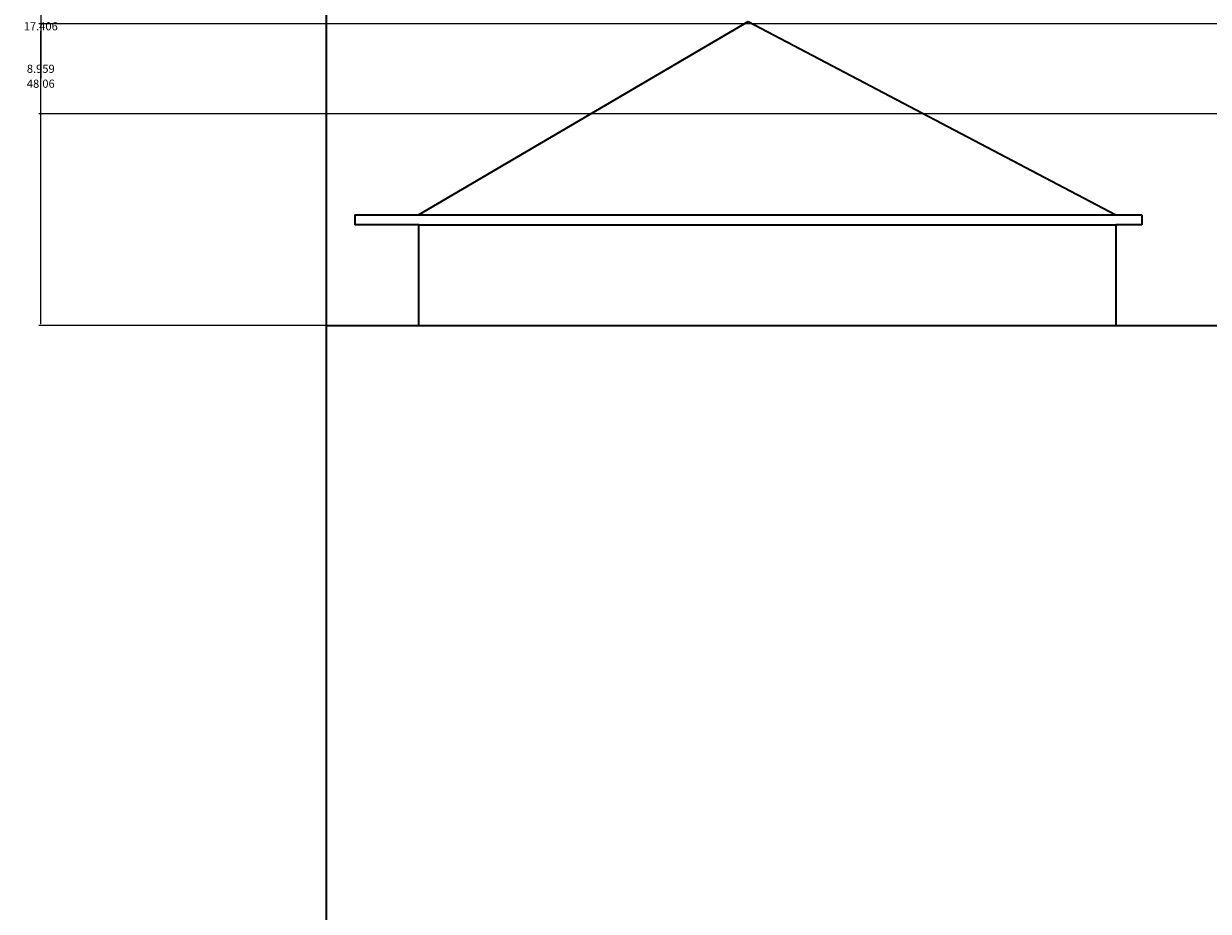
# Model space of a CAD drawing. Units: inches. Extents: x 69 to 650, y -16 to 573.
# Tile 12 of 26: x 69 to 187, y 306 to 394. Entities that reach past the tile are written whole.
import ezdxf

# ---------------------------------------------------------------- set-up
doc = ezdxf.new("R2010")
doc.units = ezdxf.units.IN
doc.header["$MEASUREMENT"] = 0
for name, color, linetype, lineweight in [('A-ANNO-DIMS', 2, 'Continuous', 18), ('A-ROOF', 7, 'Continuous', 35), ('A-WALL', 7, 'Continuous', 35)]:
    doc.layers.add(name, color=color, linetype=linetype, lineweight=lineweight)
doc.styles.get("Standard").update_dxf_attribs({"font": 'arial.ttf'})
doc.dimstyles.get("Standard").update_dxf_attribs({"dimtxt": 0.8125, "dimasz": 0.18, "dimexe": 0.18, "dimexo": 0.0625, "dimgap": 0.09, "dimtad": 0, "dimtih": 1, "dimtoh": 1, "dimdec": 4, "dimzin": 0, "dimdsep": 46, "dimlunit": 4, "dimtxsty": 'Standard', "dimcen": 0.09, "dimadec": 0, "dimazin": 0, "dimtfac": 1, "dimtdec": 4, "dimtofl": 0, "dimtmove": 0, "dimatfit": 3, "dimfxl": 1, "dimtolj": 1, "dimtzin": 0, "dimarcsym": 0})

# ---------------------------------------------------------------- blocks, each defined once
blk = doc.blocks.new('CAP-SIDE-PEDIMENT')
for p, q in [((39.09, 30.19), (2.58, 11)), ((71.85, 11), (39.09, 30.19)), ((78.18, 11), (0, 11)), ((0, 11), (0, 9.99)), ((0, 9.99), (2.58, 9.99)), ((71.82, 9.99), (2.58, 9.99)), ((2.58, 9.99), (2.58, 0)), ((71.82, 0), (71.82, 9.99)), ((71.82, 9.99), (78.18, 9.99))]:
    blk.add_line(p, q)
blk = doc.blocks.new('*D19')
at = {"layer": 'A-ANNO-DIMS', "color": 0, "lineweight": -2, "transparency": 16777216}
for p, q in [((99.56, 471.72), (99.56, 572.74)), ((99.74, 572.56), (358.57, 572.56)), ((619.38, 572.56), (360.54, 572.56)), ((619.56, 87.99), (619.56, 572.74))]:
    blk.add_line(p, q, dxfattribs=at)
at = {"layer": 'A-ANNO-DIMS', "color": 0, "transparency": 16777216}
for points in [[(99.74, 572.59), (99.74, 572.53), (99.56, 572.56)], [(619.38, 572.59), (619.38, 572.53), (619.56, 572.56)]]:
    blk.add_solid(points, dxfattribs=at)
at = {"layer": 'Defpoints', "color": 0, "transparency": 16777216}
for p in [(619.56, 572.56), (99.56, 471.66), (619.56, 87.93)]:
    blk.add_point(p, dxfattribs=at)
at = {"layer": 'A-ANNO-DIMS', "color": 0, "transparency": 16777216, "insert": (359.56, 572.56), "char_height": 0.812, "attachment_point": 5}
blk.add_mtext('\\A1;520', dxfattribs=at)
blk = doc.blocks.new('*D47')
at = {"layer": 'A-ANNO-DIMS', "color": 0, "lineweight": -2, "transparency": 16777216}
for p, q in [((99.49, 411.93), (70.98, 411.93)), ((71.16, 411.75), (71.16, 388.41)), ((71.16, 364.05), (71.16, 387.4)), ((99.49, 363.87), (70.98, 363.87))]:
    blk.add_line(p, q, dxfattribs=at)
at = {"layer": 'A-ANNO-DIMS', "color": 0, "transparency": 16777216}
for points in [[(71.13, 411.75), (71.19, 411.75), (71.16, 411.93)], [(71.13, 364.05), (71.19, 364.05), (71.16, 363.87)]]:
    blk.add_solid(points, dxfattribs=at)
at = {"layer": 'Defpoints', "color": 0, "transparency": 16777216}
for p in [(71.16, 411.93), (99.56, 411.93), (99.56, 363.87)]:
    blk.add_point(p, dxfattribs=at)
at = {"layer": 'A-ANNO-DIMS', "color": 0, "transparency": 16777216, "insert": (71.16, 387.9), "char_height": 0.812, "attachment_point": 5}
blk.add_mtext('\\A1;48.06', dxfattribs=at)
blk = doc.blocks.new('*D59')
at = {"layer": 'A-ANNO-DIMS', "color": 0, "lineweight": -2, "transparency": 16777216}
for p, q in [((214.82, 402.3), (70.98, 402.3)), ((71.16, 402.12), (71.16, 394.11)), ((71.16, 385.08), (71.16, 393.1)), ((307.73, 384.9), (70.98, 384.9))]:
    blk.add_line(p, q, dxfattribs=at)
at = {"layer": 'A-ANNO-DIMS', "color": 0, "transparency": 16777216}
for points in [[(71.13, 402.12), (71.19, 402.12), (71.16, 402.3)], [(71.13, 385.08), (71.19, 385.08), (71.16, 384.9)]]:
    blk.add_solid(points, dxfattribs=at)
at = {"layer": 'Defpoints', "color": 0, "transparency": 16777216}
for p in [(71.16, 402.3), (214.89, 402.3), (307.8, 384.9)]:
    blk.add_point(p, dxfattribs=at)
at = {"layer": 'A-ANNO-DIMS', "color": 0, "transparency": 16777216, "insert": (71.16, 393.6), "char_height": 0.812, "attachment_point": 5}
blk.add_mtext('\\A1;17.406', dxfattribs=at)
blk = doc.blocks.new('*D63')
at = {"layer": 'A-ANNO-DIMS', "color": 0, "lineweight": -2, "transparency": 16777216}
for p, q in [((319.49, 393.86), (70.98, 393.86)), ((71.16, 393.68), (71.16, 389.88)), ((71.16, 385.08), (71.16, 388.87)), ((307.73, 384.9), (70.98, 384.9))]:
    blk.add_line(p, q, dxfattribs=at)
at = {"layer": 'A-ANNO-DIMS', "color": 0, "transparency": 16777216}
for points in [[(71.13, 393.68), (71.19, 393.68), (71.16, 393.86)], [(71.13, 385.08), (71.19, 385.08), (71.16, 384.9)]]:
    blk.add_solid(points, dxfattribs=at)
at = {"layer": 'Defpoints', "color": 0, "transparency": 16777216}
for p in [(71.16, 393.86), (319.55, 393.86), (307.8, 384.9)]:
    blk.add_point(p, dxfattribs=at)
at = {"layer": 'A-ANNO-DIMS', "color": 0, "transparency": 16777216, "insert": (71.16, 389.38), "char_height": 0.812, "attachment_point": 5}
blk.add_mtext('\\A1;8.959', dxfattribs=at)

msp = doc.modelspace()

# ---------------------------------------------------------------- linework, layer by layer
at = {"layer": 'A-ROOF'}
msp.add_line((102.3654, 374.8764), (102.3654, 373.8686), dxfattribs=at)
at = {"layer": 'A-WALL'}
msp.add_line((99.556, 243.93), (99.556, 411.93), dxfattribs=at)
msp.add_lwpolyline([(99.556, 363.8739), (190.299, 363.8739), (190.299, 243.93), (99.556, 243.93)], close=True, dxfattribs=at)

# ---------------------------------------------------------------- block references
at = {"layer": 'A-ROOF', "extrusion": (0, 0, -1), "zscale": -1}
msp.add_blockref('CAP-SIDE-PEDIMENT', (-180.548, 363.874), dxfattribs=at)

# ---------------------------------------------------------------- dimensions: what is measured, and where the dimension line sits
at = {"layer": 'A-ANNO-DIMS'}
dim = msp.add_linear_dim(base=(619.555, 572.5573), p1=(99.556, 471.6595), p2=(619.555, 87.93), dimstyle='Standard', override={"dimdec": 0, "dimlfac": 1, "dimrnd": 0, "dimzin": 0, "dimdsep": 46, "dimlunit": 2}, dxfattribs=at)
dim.commit()
dim.dimension.update_dxf_attribs({"geometry": '*D19', "text_midpoint": (359.5555, 572.5573)})
for base, p1, p2, override, picture, middle in [((71.156, 411.93), (99.556, 363.8739), (99.556, 411.93), {"dimdec": 2, "dimlfac": 1, "dimrnd": 0, "dimzin": 0, "dimdsep": 46, "dimlunit": 2}, '*D47', (71.156, 387.902)), ((71.156, 402.3042), (307.7955, 384.8986), (214.8863, 402.3042), {"dimdec": 3, "dimlfac": 1, "dimrnd": 0, "dimzin": 0, "dimdsep": 46, "dimlunit": 2}, '*D59', (71.156, 393.6014)), ((71.156, 393.8576), (307.7955, 384.8986), (319.5513, 393.8576), {"dimdec": 3, "dimlfac": 1, "dimrnd": 0, "dimzin": 0, "dimdsep": 46, "dimlunit": 2}, '*D63', (71.156, 389.3781))]:
    dim = msp.add_linear_dim(base=base, p1=p1, p2=p2, angle=90, dimstyle='Standard', override=override, dxfattribs=at)
    dim.commit()
    dim.dimension.update_dxf_attribs({"geometry": picture, "text_midpoint": middle})

doc.saveas('drawing.dxf')
